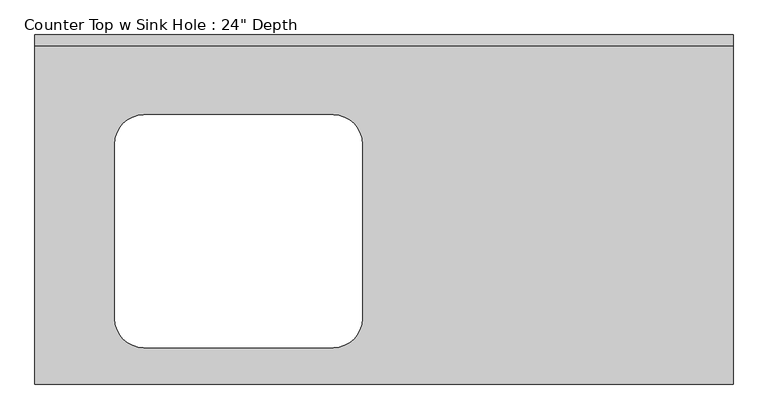
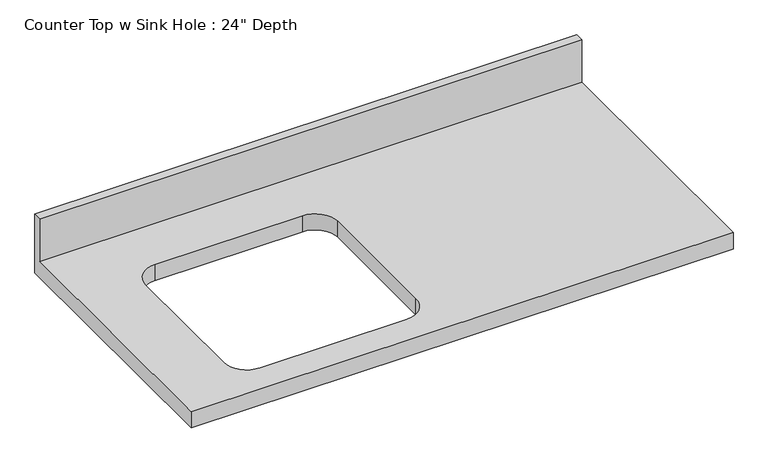
"""IFC4 building model written with IfcOpenShell, lengths in millimetres: furniture geometry."""

from ifc_helpers import new_model, si_unit, frame, origin, place, context, project, spatial, polyline, circle_curve, source, transform, mapped, element, save
from ifc_brep_helpers import plane_surface, revolved_surface, advanced_brep


def furniture_21562906(model_context):
    return source(origin(), model_context, "Body", "AdvancedBrep", [
        advanced_brep(
        [(-1200.4622951, -609.6, 914.4), (18.7377049, -609.6, 914.4), (18.7377049, -19.05, 914.4), (-1200.4622951, -19.05, 914.4), (-1009.9622951, -139.7, 914.4), (-679.7622951, -139.7, 914.4), (-628.9622951, -190.5, 914.4), (-628.9622951, -495.3, 914.4), (-679.7622951, -546.1, 914.4), (-1009.9622951, -546.1, 914.4), (-1060.7622951, -495.3, 914.4), (-1060.7622951, -190.5, 914.4), (18.7377049, 0.0, 876.3), (18.7377049, -609.6, 876.3), (-1200.4622951, -609.6, 876.3), (-1200.4622951, 0.0, 876.3), (-679.7622951, -139.7, 876.3), (-1009.9622951, -139.7, 876.3), (-1060.7622951, -190.5, 876.3), (-1060.7622951, -495.3, 876.3), (-1009.9622951, -546.1, 876.3), (-679.7622951, -546.1, 876.3), (-628.9622951, -495.3, 876.3), (-628.9622951, -190.5, 876.3), (-1200.4622951, 0.0, 1016.0), (18.7377049, 0.0, 1016.0), (-1200.4622951, -19.05, 1016.0), (18.7377049, -19.05, 1016.0)],
        [
            (0, 1),
            (1, 2),
            (2, 3),
            (3, 0),
            (4, 5),
            (5, 6, circle_curve(frame((-679.7622951, -190.5, 914.4), z_axis=(0.0, 0.0, -1.0), x_axis=(1.0, 0.0, 0.0)), 50.8)),
            (6, 7),
            (7, 8, circle_curve(frame((-679.7622951, -495.3, 914.4), z_axis=(0.0, 0.0, -1.0), x_axis=(1.0, 0.0, 0.0)), 50.8)),
            (8, 9),
            (9, 10, circle_curve(frame((-1009.9622951, -495.3, 914.4), z_axis=(0.0, 0.0, -1.0), x_axis=(1.0, 0.0, 0.0)), 50.8)),
            (10, 11),
            (11, 4, circle_curve(frame((-1009.9622951, -190.5, 914.4), z_axis=(0.0, 0.0, -1.0), x_axis=(1.0, 0.0, 0.0)), 50.8)),
            (12, 13),
            (13, 14),
            (14, 15),
            (15, 12),
            (16, 17),
            (17, 18, circle_curve(frame((-1009.9622951, -190.5, 876.3), z_axis=(0.0, 0.0, 1.0), x_axis=(1.0, 0.0, 0.0)), 50.8)),
            (18, 19),
            (19, 20, circle_curve(frame((-1009.9622951, -495.3, 876.3), z_axis=(0.0, 0.0, 1.0), x_axis=(1.0, 0.0, 0.0)), 50.8)),
            (20, 21),
            (21, 22, circle_curve(frame((-679.7622951, -495.3, 876.3), z_axis=(0.0, 0.0, 1.0), x_axis=(1.0, 0.0, 0.0)), 50.8)),
            (22, 23),
            (23, 16, circle_curve(frame((-679.7622951, -190.5, 876.3), z_axis=(0.0, 0.0, 1.0), x_axis=(1.0, 0.0, 0.0)), 50.8)),
            (15, 24),
            (24, 25),
            (25, 12),
            (14, 0),
            (3, 26),
            (26, 24),
            (13, 1),
            (25, 27),
            (27, 2),
            (4, 17),
            (16, 5),
            (11, 18),
            (10, 19),
            (9, 20),
            (8, 21),
            (7, 22),
            (6, 23),
            (26, 27),
        ],
        [
            plane_surface(frame((-1200.4622951, 0.0, 914.4), z_axis=(0.0, 0.0, 1.0), x_axis=(-1.0, 0.0, 0.0))),
            plane_surface(frame((-1200.4622951, 0.0, 876.3), z_axis=(0.0, 0.0, -1.0), x_axis=(1.0, 0.0, 0.0))),
            plane_surface(frame((18.7377049, 0.0, 914.4), z_axis=(0.0, 1.0, 0.0), x_axis=(0.0, 0.0, -1.0))),
            plane_surface(frame((-1200.4622951, 0.0, 914.4), z_axis=(-1.0, 0.0, 0.0), x_axis=(0.0, 0.0, -1.0))),
            plane_surface(frame((-1200.4622951, -609.6, 914.4), z_axis=(0.0, -1.0, 0.0), x_axis=(0.0, 0.0, -1.0))),
            plane_surface(frame((18.7377049, -609.6, 914.4), z_axis=(1.0, 0.0, 0.0), x_axis=(0.0, 0.0, -1.0))),
            plane_surface(frame((-679.7622951, -139.7, 914.4), z_axis=(0.0, -1.0, 0.0), x_axis=(0.0, 0.0, -1.0))),
            revolved_surface(polyline([(-959.1622951, -190.5, 914.4), (-959.1622951, -190.5, 876.3)]), (-1009.9622951, -190.5, 876.3), (0.0, 0.0, 1.0)),
            plane_surface(frame((-1060.7622951, -190.5, 914.4), z_axis=(1.0, 0.0, 0.0), x_axis=(0.0, 0.0, -1.0))),
            revolved_surface(polyline([(-959.1622951, -495.3, 914.4), (-959.1622951, -495.3, 876.3)]), (-1009.9622951, -495.3, 876.3), (0.0, 0.0, 1.0)),
            plane_surface(frame((-1009.9622951, -546.1, 914.4), z_axis=(0.0, 1.0, 0.0), x_axis=(0.0, 0.0, -1.0))),
            revolved_surface(polyline([(-628.9622951, -495.3, 914.4), (-628.9622951, -495.3, 876.3)]), (-679.7622951, -495.3, 876.3), (0.0, 0.0, 1.0)),
            plane_surface(frame((-628.9622951, -495.3, 914.4), z_axis=(-1.0, 0.0, 0.0), x_axis=(0.0, 0.0, -1.0))),
            revolved_surface(polyline([(-628.9622951, -190.5, 914.4), (-628.9622951, -190.5, 876.3)]), (-679.7622951, -190.5, 876.3), (0.0, 0.0, 1.0)),
            plane_surface(frame((-1200.4622951, 0.0, 1016.0), z_axis=(0.0, 0.0, 1.0), x_axis=(0.0, -1.0, 0.0))),
            plane_surface(frame((-1200.4622951, -19.05, 1016.0), z_axis=(0.0, -1.0, 0.0), x_axis=(0.0, 0.0, -1.0))),
        ],
        [
            (0, [[1, 2, 3, 4], [5, 6, 7, 8, 9, 10, 11, 12]]),
            (1, [[13, 14, 15, 16], [17, 18, 19, 20, 21, 22, 23, 24]]),
            (2, [[-16, 25, 26, 27]]),
            (3, [[-15, 28, -4, 29, 30, -25]]),
            (4, [[-1, -28, -14, 31]]),
            (5, [[-13, -27, 32, 33, -2, -31]]),
            (6, [[34, -17, 35, -5]]),
            (7, [[-34, -12, 36, -18]]),
            (8, [[-36, -11, 37, -19]]),
            (9, [[-37, -10, 38, -20]]),
            (10, [[-38, -9, 39, -21]]),
            (11, [[-39, -8, 40, -22]]),
            (12, [[-40, -7, 41, -23]]),
            (13, [[-35, -24, -41, -6]]),
            (14, [[-30, 42, -32, -26]]),
            (15, [[-42, -29, -3, -33]]),
        ],
    ),
    ])


if __name__ == "__main__":
    model = new_model("IFC4")
    model_context = context("Model", 3, world=origin())
    ifc_project = project(units=[si_unit("LENGTHUNIT", "METRE", prefix="MILLI")], contexts=[model_context])
    site = spatial("IfcSite", under=ifc_project)
    building = spatial("IfcBuilding", under=site)
    placement = place(None, origin())
    furniture_shape = furniture_21562906(model_context)
    element("IfcFurniture", 1, ObjectType="Counter Top w Sink Hole : 24\" Depth", at=placement, inside=building, context=model_context, shape_type="MappedRepresentation", body=[
        mapped(furniture_shape, transform((0.0, 0.0, 0.0), x_axis=(1.0, 0.0, 0.0), y_axis=(0.0, 1.0, 0.0), z_axis=(0.0, 0.0, 1.0))),
    ])
    save(model, "model.ifc")

# Revit data of these elements
# Type "Counter Top w Sink Hole : 24\" Depth"
#   Assembly Code = "C1030400"
#   Counter Thickness = 0' - 1 1/2"
#   Depth [instance default] = 2' - 1"
#   Height = 3' - 0"
#   Length [instance default] = 8' - 0"
#   Sink Location [instance default] = 2' - 0"
#   Sink Location To Wall [instance default] = 0' - 6"
#   Sink Opening Depth [instance default] = 1' - 3"
#   Sink Opening Width [instance default] = 2' - 3"
#   Counter Top Material = none
#   Default Elevation = 0
# Element 1 (IfcFurniture, "Counter Top w Sink Hole : 24\" Depth")
#   Depth = 2' - 0"
#   Length = 4' - 0"
#   Sink Location = 1' - 2"
#   Sink Opening Width = 1' - 4"
#   Materials on its faces: "Counter Top"
# Materials
#   "Counter Top": class "Wood", colour RGB 226 177 128, transparency 0
